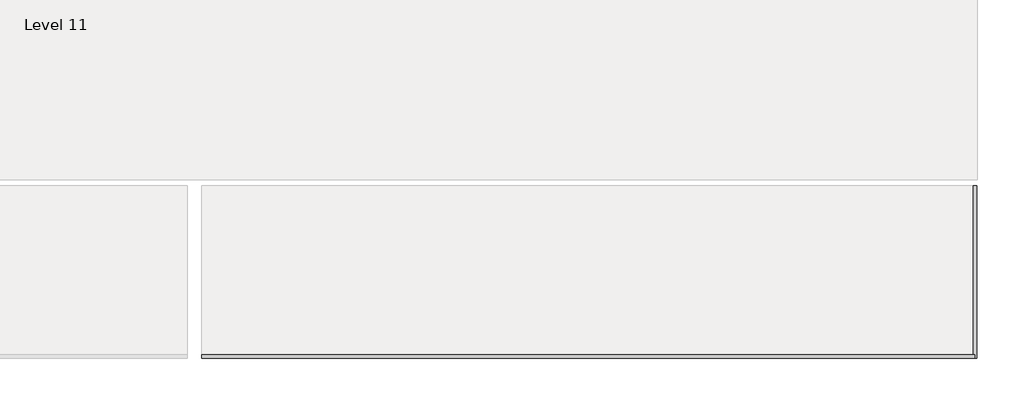
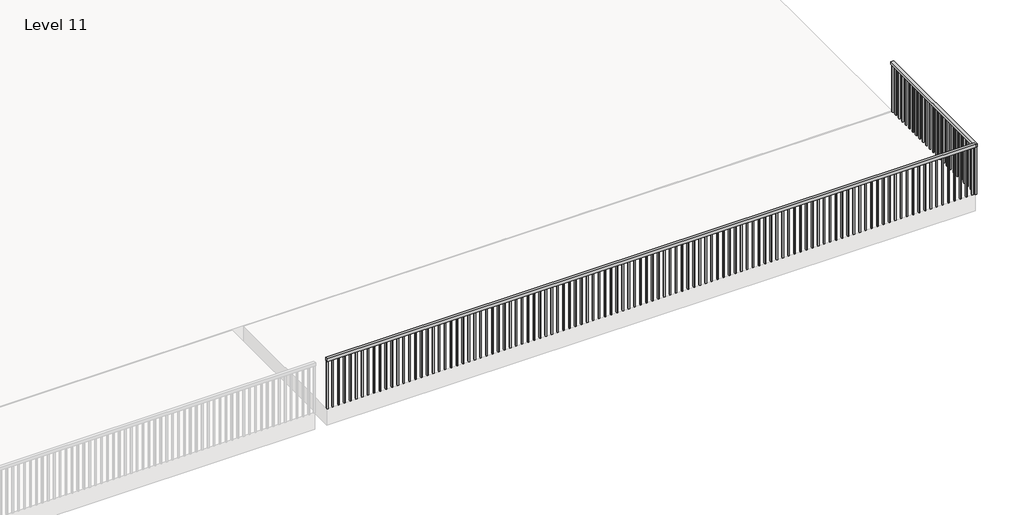
# One storey, part 2 of 5: 2 railings.
"""IFC4 building model written with IfcOpenShell, lengths in millimetres."""

from ifc_helpers import new_model, si_unit, frame, origin, place, context, project, spatial, polyline, outline, extrude, element, save

model = new_model("IFC4")

# Units and contexts
model_context = context("Model", 3, world=origin())
ifc_project = project(units=[si_unit("LENGTHUNIT", "METRE", prefix="MILLI")], contexts=[model_context])

# Site, building, storey
site = spatial("IfcSite", under=ifc_project)
building = spatial("IfcBuilding", under=site)
storey = spatial("IfcBuildingStorey", under=building, Name="Level 11", Elevation=15544.8)

# Railings
placement = place(None, origin())
element("IfcRailing", 1, ObjectType="Handrail - Rectangular", at=placement, inside=storey, context=model_context, shape_type="SweptSolid", body=[
    extrude(outline(polyline([(2981.3361222, -12911.7749501), (2981.3361222, -12860.9749501), (14106.5361222, -12860.9749501), (14106.5361222, -12911.7749501), (2981.3361222, -12911.7749501)])), frame((0.0, 0.0, 16408.4), z_axis=(0.0, 0.0, 1.0), x_axis=(1.0, 0.0, 0.0)), (0.0, 0.0, 1.0), 50.8),
    extrude(outline(polyline([(14046.2111222, -12895.8999501), (14046.2111222, -12876.8499501), (14065.2611222, -12876.8499501), (14065.2611222, -12895.8999501), (14046.2111222, -12895.8999501)])), frame((0.0, 0.0, 15544.8), z_axis=(0.0, 0.0, 1.0), x_axis=(1.0, 0.0, 0.0)), (0.0, 0.0, 1.0), 863.6),
    extrude(outline(polyline([(13944.6111222, -12895.8999501), (13944.6111222, -12876.8499501), (13963.6611222, -12876.8499501), (13963.6611222, -12895.8999501), (13944.6111222, -12895.8999501)])), frame((0.0, 0.0, 15544.8), z_axis=(0.0, 0.0, 1.0), x_axis=(1.0, 0.0, 0.0)), (0.0, 0.0, 1.0), 863.6),
    extrude(outline(polyline([(13843.0111222, -12895.8999501), (13843.0111222, -12876.8499501), (13862.0611222, -12876.8499501), (13862.0611222, -12895.8999501), (13843.0111222, -12895.8999501)])), frame((0.0, 0.0, 15544.8), z_axis=(0.0, 0.0, 1.0), x_axis=(1.0, 0.0, 0.0)), (0.0, 0.0, 1.0), 863.6),
    extrude(outline(polyline([(13741.4111222, -12895.8999501), (13741.4111222, -12876.8499501), (13760.4611222, -12876.8499501), (13760.4611222, -12895.8999501), (13741.4111222, -12895.8999501)])), frame((0.0, 0.0, 15544.8), z_axis=(0.0, 0.0, 1.0), x_axis=(1.0, 0.0, 0.0)), (0.0, 0.0, 1.0), 863.6),
    extrude(outline(polyline([(13639.8111222, -12895.8999501), (13639.8111222, -12876.8499501), (13658.8611222, -12876.8499501), (13658.8611222, -12895.8999501), (13639.8111222, -12895.8999501)])), frame((0.0, 0.0, 15544.8), z_axis=(0.0, 0.0, 1.0), x_axis=(1.0, 0.0, 0.0)), (0.0, 0.0, 1.0), 863.6),
    extrude(outline(polyline([(13538.2111222, -12895.8999501), (13538.2111222, -12876.8499501), (13557.2611222, -12876.8499501), (13557.2611222, -12895.8999501), (13538.2111222, -12895.8999501)])), frame((0.0, 0.0, 15544.8), z_axis=(0.0, 0.0, 1.0), x_axis=(1.0, 0.0, 0.0)), (0.0, 0.0, 1.0), 863.6),
    extrude(outline(polyline([(13436.6111222, -12895.8999501), (13436.6111222, -12876.8499501), (13455.6611222, -12876.8499501), (13455.6611222, -12895.8999501), (13436.6111222, -12895.8999501)])), frame((0.0, 0.0, 15544.8), z_axis=(0.0, 0.0, 1.0), x_axis=(1.0, 0.0, 0.0)), (0.0, 0.0, 1.0), 863.6),
    extrude(outline(polyline([(13335.0111222, -12895.8999501), (13335.0111222, -12876.8499501), (13354.0611222, -12876.8499501), (13354.0611222, -12895.8999501), (13335.0111222, -12895.8999501)])), frame((0.0, 0.0, 15544.8), z_axis=(0.0, 0.0, 1.0), x_axis=(1.0, 0.0, 0.0)), (0.0, 0.0, 1.0), 863.6),
    extrude(outline(polyline([(13233.4111222, -12895.8999501), (13233.4111222, -12876.8499501), (13252.4611222, -12876.8499501), (13252.4611222, -12895.8999501), (13233.4111222, -12895.8999501)])), frame((0.0, 0.0, 15544.8), z_axis=(0.0, 0.0, 1.0), x_axis=(1.0, 0.0, 0.0)), (0.0, 0.0, 1.0), 863.6),
    extrude(outline(polyline([(13131.8111222, -12895.8999501), (13131.8111222, -12876.8499501), (13150.8611222, -12876.8499501), (13150.8611222, -12895.8999501), (13131.8111222, -12895.8999501)])), frame((0.0, 0.0, 15544.8), z_axis=(0.0, 0.0, 1.0), x_axis=(1.0, 0.0, 0.0)), (0.0, 0.0, 1.0), 863.6),
    extrude(outline(polyline([(13030.2111222, -12895.8999501), (13030.2111222, -12876.8499501), (13049.2611222, -12876.8499501), (13049.2611222, -12895.8999501), (13030.2111222, -12895.8999501)])), frame((0.0, 0.0, 15544.8), z_axis=(0.0, 0.0, 1.0), x_axis=(1.0, 0.0, 0.0)), (0.0, 0.0, 1.0), 863.6),
    extrude(outline(polyline([(12928.6111222, -12895.8999501), (12928.6111222, -12876.8499501), (12947.6611222, -12876.8499501), (12947.6611222, -12895.8999501), (12928.6111222, -12895.8999501)])), frame((0.0, 0.0, 15544.8), z_axis=(0.0, 0.0, 1.0), x_axis=(1.0, 0.0, 0.0)), (0.0, 0.0, 1.0), 863.6),
    extrude(outline(polyline([(12827.0111222, -12895.8999501), (12827.0111222, -12876.8499501), (12846.0611222, -12876.8499501), (12846.0611222, -12895.8999501), (12827.0111222, -12895.8999501)])), frame((0.0, 0.0, 15544.8), z_axis=(0.0, 0.0, 1.0), x_axis=(1.0, 0.0, 0.0)), (0.0, 0.0, 1.0), 863.6),
    extrude(outline(polyline([(12725.4111222, -12895.8999501), (12725.4111222, -12876.8499501), (12744.4611222, -12876.8499501), (12744.4611222, -12895.8999501), (12725.4111222, -12895.8999501)])), frame((0.0, 0.0, 15544.8), z_axis=(0.0, 0.0, 1.0), x_axis=(1.0, 0.0, 0.0)), (0.0, 0.0, 1.0), 863.6),
    extrude(outline(polyline([(12623.8111222, -12895.8999501), (12623.8111222, -12876.8499501), (12642.8611222, -12876.8499501), (12642.8611222, -12895.8999501), (12623.8111222, -12895.8999501)])), frame((0.0, 0.0, 15544.8), z_axis=(0.0, 0.0, 1.0), x_axis=(1.0, 0.0, 0.0)), (0.0, 0.0, 1.0), 863.6),
    extrude(outline(polyline([(12522.2111222, -12895.8999501), (12522.2111222, -12876.8499501), (12541.2611222, -12876.8499501), (12541.2611222, -12895.8999501), (12522.2111222, -12895.8999501)])), frame((0.0, 0.0, 15544.8), z_axis=(0.0, 0.0, 1.0), x_axis=(1.0, 0.0, 0.0)), (0.0, 0.0, 1.0), 863.6),
    extrude(outline(polyline([(12420.6111222, -12895.8999501), (12420.6111222, -12876.8499501), (12439.6611222, -12876.8499501), (12439.6611222, -12895.8999501), (12420.6111222, -12895.8999501)])), frame((0.0, 0.0, 15544.8), z_axis=(0.0, 0.0, 1.0), x_axis=(1.0, 0.0, 0.0)), (0.0, 0.0, 1.0), 863.6),
    extrude(outline(polyline([(12319.0111222, -12895.8999501), (12319.0111222, -12876.8499501), (12338.0611222, -12876.8499501), (12338.0611222, -12895.8999501), (12319.0111222, -12895.8999501)])), frame((0.0, 0.0, 15544.8), z_axis=(0.0, 0.0, 1.0), x_axis=(1.0, 0.0, 0.0)), (0.0, 0.0, 1.0), 863.6),
    extrude(outline(polyline([(12217.4111222, -12895.8999501), (12217.4111222, -12876.8499501), (12236.4611222, -12876.8499501), (12236.4611222, -12895.8999501), (12217.4111222, -12895.8999501)])), frame((0.0, 0.0, 15544.8), z_axis=(0.0, 0.0, 1.0), x_axis=(1.0, 0.0, 0.0)), (0.0, 0.0, 1.0), 863.6),
    extrude(outline(polyline([(12115.8111222, -12895.8999501), (12115.8111222, -12876.8499501), (12134.8611222, -12876.8499501), (12134.8611222, -12895.8999501), (12115.8111222, -12895.8999501)])), frame((0.0, 0.0, 15544.8), z_axis=(0.0, 0.0, 1.0), x_axis=(1.0, 0.0, 0.0)), (0.0, 0.0, 1.0), 863.6),
    extrude(outline(polyline([(12014.2111222, -12895.8999501), (12014.2111222, -12876.8499501), (12033.2611222, -12876.8499501), (12033.2611222, -12895.8999501), (12014.2111222, -12895.8999501)])), frame((0.0, 0.0, 15544.8), z_axis=(0.0, 0.0, 1.0), x_axis=(1.0, 0.0, 0.0)), (0.0, 0.0, 1.0), 863.6),
    extrude(outline(polyline([(11912.6111222, -12895.8999501), (11912.6111222, -12876.8499501), (11931.6611222, -12876.8499501), (11931.6611222, -12895.8999501), (11912.6111222, -12895.8999501)])), frame((0.0, 0.0, 15544.8), z_axis=(0.0, 0.0, 1.0), x_axis=(1.0, 0.0, 0.0)), (0.0, 0.0, 1.0), 863.6),
    extrude(outline(polyline([(11811.0111222, -12895.8999501), (11811.0111222, -12876.8499501), (11830.0611222, -12876.8499501), (11830.0611222, -12895.8999501), (11811.0111222, -12895.8999501)])), frame((0.0, 0.0, 15544.8), z_axis=(0.0, 0.0, 1.0), x_axis=(1.0, 0.0, 0.0)), (0.0, 0.0, 1.0), 863.6),
    extrude(outline(polyline([(11709.4111222, -12895.8999501), (11709.4111222, -12876.8499501), (11728.4611222, -12876.8499501), (11728.4611222, -12895.8999501), (11709.4111222, -12895.8999501)])), frame((0.0, 0.0, 15544.8), z_axis=(0.0, 0.0, 1.0), x_axis=(1.0, 0.0, 0.0)), (0.0, 0.0, 1.0), 863.6),
    extrude(outline(polyline([(11607.8111222, -12895.8999501), (11607.8111222, -12876.8499501), (11626.8611222, -12876.8499501), (11626.8611222, -12895.8999501), (11607.8111222, -12895.8999501)])), frame((0.0, 0.0, 15544.8), z_axis=(0.0, 0.0, 1.0), x_axis=(1.0, 0.0, 0.0)), (0.0, 0.0, 1.0), 863.6),
    extrude(outline(polyline([(11506.2111222, -12895.8999501), (11506.2111222, -12876.8499501), (11525.2611222, -12876.8499501), (11525.2611222, -12895.8999501), (11506.2111222, -12895.8999501)])), frame((0.0, 0.0, 15544.8), z_axis=(0.0, 0.0, 1.0), x_axis=(1.0, 0.0, 0.0)), (0.0, 0.0, 1.0), 863.6),
    extrude(outline(polyline([(11404.6111222, -12895.8999501), (11404.6111222, -12876.8499501), (11423.6611222, -12876.8499501), (11423.6611222, -12895.8999501), (11404.6111222, -12895.8999501)])), frame((0.0, 0.0, 15544.8), z_axis=(0.0, 0.0, 1.0), x_axis=(1.0, 0.0, 0.0)), (0.0, 0.0, 1.0), 863.6),
    extrude(outline(polyline([(11303.0111222, -12895.8999501), (11303.0111222, -12876.8499501), (11322.0611222, -12876.8499501), (11322.0611222, -12895.8999501), (11303.0111222, -12895.8999501)])), frame((0.0, 0.0, 15544.8), z_axis=(0.0, 0.0, 1.0), x_axis=(1.0, 0.0, 0.0)), (0.0, 0.0, 1.0), 863.6),
    extrude(outline(polyline([(11201.4111222, -12895.8999501), (11201.4111222, -12876.8499501), (11220.4611222, -12876.8499501), (11220.4611222, -12895.8999501), (11201.4111222, -12895.8999501)])), frame((0.0, 0.0, 15544.8), z_axis=(0.0, 0.0, 1.0), x_axis=(1.0, 0.0, 0.0)), (0.0, 0.0, 1.0), 863.6),
    extrude(outline(polyline([(11099.8111222, -12895.8999501), (11099.8111222, -12876.8499501), (11118.8611222, -12876.8499501), (11118.8611222, -12895.8999501), (11099.8111222, -12895.8999501)])), frame((0.0, 0.0, 15544.8), z_axis=(0.0, 0.0, 1.0), x_axis=(1.0, 0.0, 0.0)), (0.0, 0.0, 1.0), 863.6),
    extrude(outline(polyline([(10998.2111222, -12895.8999501), (10998.2111222, -12876.8499501), (11017.2611222, -12876.8499501), (11017.2611222, -12895.8999501), (10998.2111222, -12895.8999501)])), frame((0.0, 0.0, 15544.8), z_axis=(0.0, 0.0, 1.0), x_axis=(1.0, 0.0, 0.0)), (0.0, 0.0, 1.0), 863.6),
    extrude(outline(polyline([(10896.6111222, -12895.8999501), (10896.6111222, -12876.8499501), (10915.6611222, -12876.8499501), (10915.6611222, -12895.8999501), (10896.6111222, -12895.8999501)])), frame((0.0, 0.0, 15544.8), z_axis=(0.0, 0.0, 1.0), x_axis=(1.0, 0.0, 0.0)), (0.0, 0.0, 1.0), 863.6),
    extrude(outline(polyline([(10795.0111222, -12895.8999501), (10795.0111222, -12876.8499501), (10814.0611222, -12876.8499501), (10814.0611222, -12895.8999501), (10795.0111222, -12895.8999501)])), frame((0.0, 0.0, 15544.8), z_axis=(0.0, 0.0, 1.0), x_axis=(1.0, 0.0, 0.0)), (0.0, 0.0, 1.0), 863.6),
    extrude(outline(polyline([(10693.4111222, -12895.8999501), (10693.4111222, -12876.8499501), (10712.4611222, -12876.8499501), (10712.4611222, -12895.8999501), (10693.4111222, -12895.8999501)])), frame((0.0, 0.0, 15544.8), z_axis=(0.0, 0.0, 1.0), x_axis=(1.0, 0.0, 0.0)), (0.0, 0.0, 1.0), 863.6),
    extrude(outline(polyline([(10591.8111222, -12895.8999501), (10591.8111222, -12876.8499501), (10610.8611222, -12876.8499501), (10610.8611222, -12895.8999501), (10591.8111222, -12895.8999501)])), frame((0.0, 0.0, 15544.8), z_axis=(0.0, 0.0, 1.0), x_axis=(1.0, 0.0, 0.0)), (0.0, 0.0, 1.0), 863.6),
    extrude(outline(polyline([(10490.2111222, -12895.8999501), (10490.2111222, -12876.8499501), (10509.2611222, -12876.8499501), (10509.2611222, -12895.8999501), (10490.2111222, -12895.8999501)])), frame((0.0, 0.0, 15544.8), z_axis=(0.0, 0.0, 1.0), x_axis=(1.0, 0.0, 0.0)), (0.0, 0.0, 1.0), 863.6),
    extrude(outline(polyline([(10388.6111222, -12895.8999501), (10388.6111222, -12876.8499501), (10407.6611222, -12876.8499501), (10407.6611222, -12895.8999501), (10388.6111222, -12895.8999501)])), frame((0.0, 0.0, 15544.8), z_axis=(0.0, 0.0, 1.0), x_axis=(1.0, 0.0, 0.0)), (0.0, 0.0, 1.0), 863.6),
    extrude(outline(polyline([(10287.0111222, -12895.8999501), (10287.0111222, -12876.8499501), (10306.0611222, -12876.8499501), (10306.0611222, -12895.8999501), (10287.0111222, -12895.8999501)])), frame((0.0, 0.0, 15544.8), z_axis=(0.0, 0.0, 1.0), x_axis=(1.0, 0.0, 0.0)), (0.0, 0.0, 1.0), 863.6),
    extrude(outline(polyline([(10185.4111222, -12895.8999501), (10185.4111222, -12876.8499501), (10204.4611222, -12876.8499501), (10204.4611222, -12895.8999501), (10185.4111222, -12895.8999501)])), frame((0.0, 0.0, 15544.8), z_axis=(0.0, 0.0, 1.0), x_axis=(1.0, 0.0, 0.0)), (0.0, 0.0, 1.0), 863.6),
    extrude(outline(polyline([(10083.8111222, -12895.8999501), (10083.8111222, -12876.8499501), (10102.8611222, -12876.8499501), (10102.8611222, -12895.8999501), (10083.8111222, -12895.8999501)])), frame((0.0, 0.0, 15544.8), z_axis=(0.0, 0.0, 1.0), x_axis=(1.0, 0.0, 0.0)), (0.0, 0.0, 1.0), 863.6),
    extrude(outline(polyline([(9982.2111222, -12895.8999501), (9982.2111222, -12876.8499501), (10001.2611222, -12876.8499501), (10001.2611222, -12895.8999501), (9982.2111222, -12895.8999501)])), frame((0.0, 0.0, 15544.8), z_axis=(0.0, 0.0, 1.0), x_axis=(1.0, 0.0, 0.0)), (0.0, 0.0, 1.0), 863.6),
    extrude(outline(polyline([(9880.6111222, -12895.8999501), (9880.6111222, -12876.8499501), (9899.6611222, -12876.8499501), (9899.6611222, -12895.8999501), (9880.6111222, -12895.8999501)])), frame((0.0, 0.0, 15544.8), z_axis=(0.0, 0.0, 1.0), x_axis=(1.0, 0.0, 0.0)), (0.0, 0.0, 1.0), 863.6),
    extrude(outline(polyline([(9779.0111222, -12895.8999501), (9779.0111222, -12876.8499501), (9798.0611222, -12876.8499501), (9798.0611222, -12895.8999501), (9779.0111222, -12895.8999501)])), frame((0.0, 0.0, 15544.8), z_axis=(0.0, 0.0, 1.0), x_axis=(1.0, 0.0, 0.0)), (0.0, 0.0, 1.0), 863.6),
    extrude(outline(polyline([(9677.4111222, -12895.8999501), (9677.4111222, -12876.8499501), (9696.4611222, -12876.8499501), (9696.4611222, -12895.8999501), (9677.4111222, -12895.8999501)])), frame((0.0, 0.0, 15544.8), z_axis=(0.0, 0.0, 1.0), x_axis=(1.0, 0.0, 0.0)), (0.0, 0.0, 1.0), 863.6),
    extrude(outline(polyline([(9575.8111222, -12895.8999501), (9575.8111222, -12876.8499501), (9594.8611222, -12876.8499501), (9594.8611222, -12895.8999501), (9575.8111222, -12895.8999501)])), frame((0.0, 0.0, 15544.8), z_axis=(0.0, 0.0, 1.0), x_axis=(1.0, 0.0, 0.0)), (0.0, 0.0, 1.0), 863.6),
    extrude(outline(polyline([(9474.2111222, -12895.8999501), (9474.2111222, -12876.8499501), (9493.2611222, -12876.8499501), (9493.2611222, -12895.8999501), (9474.2111222, -12895.8999501)])), frame((0.0, 0.0, 15544.8), z_axis=(0.0, 0.0, 1.0), x_axis=(1.0, 0.0, 0.0)), (0.0, 0.0, 1.0), 863.6),
    extrude(outline(polyline([(9372.6111222, -12895.8999501), (9372.6111222, -12876.8499501), (9391.6611222, -12876.8499501), (9391.6611222, -12895.8999501), (9372.6111222, -12895.8999501)])), frame((0.0, 0.0, 15544.8), z_axis=(0.0, 0.0, 1.0), x_axis=(1.0, 0.0, 0.0)), (0.0, 0.0, 1.0), 863.6),
    extrude(outline(polyline([(9271.0111222, -12895.8999501), (9271.0111222, -12876.8499501), (9290.0611222, -12876.8499501), (9290.0611222, -12895.8999501), (9271.0111222, -12895.8999501)])), frame((0.0, 0.0, 15544.8), z_axis=(0.0, 0.0, 1.0), x_axis=(1.0, 0.0, 0.0)), (0.0, 0.0, 1.0), 863.6),
    extrude(outline(polyline([(9169.4111222, -12895.8999501), (9169.4111222, -12876.8499501), (9188.4611222, -12876.8499501), (9188.4611222, -12895.8999501), (9169.4111222, -12895.8999501)])), frame((0.0, 0.0, 15544.8), z_axis=(0.0, 0.0, 1.0), x_axis=(1.0, 0.0, 0.0)), (0.0, 0.0, 1.0), 863.6),
    extrude(outline(polyline([(9067.8111222, -12895.8999501), (9067.8111222, -12876.8499501), (9086.8611222, -12876.8499501), (9086.8611222, -12895.8999501), (9067.8111222, -12895.8999501)])), frame((0.0, 0.0, 15544.8), z_axis=(0.0, 0.0, 1.0), x_axis=(1.0, 0.0, 0.0)), (0.0, 0.0, 1.0), 863.6),
    extrude(outline(polyline([(8966.2111222, -12895.8999501), (8966.2111222, -12876.8499501), (8985.2611222, -12876.8499501), (8985.2611222, -12895.8999501), (8966.2111222, -12895.8999501)])), frame((0.0, 0.0, 15544.8), z_axis=(0.0, 0.0, 1.0), x_axis=(1.0, 0.0, 0.0)), (0.0, 0.0, 1.0), 863.6),
    extrude(outline(polyline([(8864.6111222, -12895.8999501), (8864.6111222, -12876.8499501), (8883.6611222, -12876.8499501), (8883.6611222, -12895.8999501), (8864.6111222, -12895.8999501)])), frame((0.0, 0.0, 15544.8), z_axis=(0.0, 0.0, 1.0), x_axis=(1.0, 0.0, 0.0)), (0.0, 0.0, 1.0), 863.6),
    extrude(outline(polyline([(8763.0111222, -12895.8999501), (8763.0111222, -12876.8499501), (8782.0611222, -12876.8499501), (8782.0611222, -12895.8999501), (8763.0111222, -12895.8999501)])), frame((0.0, 0.0, 15544.8), z_axis=(0.0, 0.0, 1.0), x_axis=(1.0, 0.0, 0.0)), (0.0, 0.0, 1.0), 863.6),
    extrude(outline(polyline([(8661.4111222, -12895.8999501), (8661.4111222, -12876.8499501), (8680.4611222, -12876.8499501), (8680.4611222, -12895.8999501), (8661.4111222, -12895.8999501)])), frame((0.0, 0.0, 15544.8), z_axis=(0.0, 0.0, 1.0), x_axis=(1.0, 0.0, 0.0)), (0.0, 0.0, 1.0), 863.6),
    extrude(outline(polyline([(8559.8111222, -12895.8999501), (8559.8111222, -12876.8499501), (8578.8611222, -12876.8499501), (8578.8611222, -12895.8999501), (8559.8111222, -12895.8999501)])), frame((0.0, 0.0, 15544.8), z_axis=(0.0, 0.0, 1.0), x_axis=(1.0, 0.0, 0.0)), (0.0, 0.0, 1.0), 863.6),
    extrude(outline(polyline([(8458.2111222, -12895.8999501), (8458.2111222, -12876.8499501), (8477.2611222, -12876.8499501), (8477.2611222, -12895.8999501), (8458.2111222, -12895.8999501)])), frame((0.0, 0.0, 15544.8), z_axis=(0.0, 0.0, 1.0), x_axis=(1.0, 0.0, 0.0)), (0.0, 0.0, 1.0), 863.6),
    extrude(outline(polyline([(8356.6111222, -12895.8999501), (8356.6111222, -12876.8499501), (8375.6611222, -12876.8499501), (8375.6611222, -12895.8999501), (8356.6111222, -12895.8999501)])), frame((0.0, 0.0, 15544.8), z_axis=(0.0, 0.0, 1.0), x_axis=(1.0, 0.0, 0.0)), (0.0, 0.0, 1.0), 863.6),
    extrude(outline(polyline([(8255.0111222, -12895.8999501), (8255.0111222, -12876.8499501), (8274.0611222, -12876.8499501), (8274.0611222, -12895.8999501), (8255.0111222, -12895.8999501)])), frame((0.0, 0.0, 15544.8), z_axis=(0.0, 0.0, 1.0), x_axis=(1.0, 0.0, 0.0)), (0.0, 0.0, 1.0), 863.6),
    extrude(outline(polyline([(8153.4111222, -12895.8999501), (8153.4111222, -12876.8499501), (8172.4611222, -12876.8499501), (8172.4611222, -12895.8999501), (8153.4111222, -12895.8999501)])), frame((0.0, 0.0, 15544.8), z_axis=(0.0, 0.0, 1.0), x_axis=(1.0, 0.0, 0.0)), (0.0, 0.0, 1.0), 863.6),
    extrude(outline(polyline([(8051.8111222, -12895.8999501), (8051.8111222, -12876.8499501), (8070.8611222, -12876.8499501), (8070.8611222, -12895.8999501), (8051.8111222, -12895.8999501)])), frame((0.0, 0.0, 15544.8), z_axis=(0.0, 0.0, 1.0), x_axis=(1.0, 0.0, 0.0)), (0.0, 0.0, 1.0), 863.6),
    extrude(outline(polyline([(7950.2111222, -12895.8999501), (7950.2111222, -12876.8499501), (7969.2611222, -12876.8499501), (7969.2611222, -12895.8999501), (7950.2111222, -12895.8999501)])), frame((0.0, 0.0, 15544.8), z_axis=(0.0, 0.0, 1.0), x_axis=(1.0, 0.0, 0.0)), (0.0, 0.0, 1.0), 863.6),
    extrude(outline(polyline([(7848.6111222, -12895.8999501), (7848.6111222, -12876.8499501), (7867.6611222, -12876.8499501), (7867.6611222, -12895.8999501), (7848.6111222, -12895.8999501)])), frame((0.0, 0.0, 15544.8), z_axis=(0.0, 0.0, 1.0), x_axis=(1.0, 0.0, 0.0)), (0.0, 0.0, 1.0), 863.6),
    extrude(outline(polyline([(7747.0111222, -12895.8999501), (7747.0111222, -12876.8499501), (7766.0611222, -12876.8499501), (7766.0611222, -12895.8999501), (7747.0111222, -12895.8999501)])), frame((0.0, 0.0, 15544.8), z_axis=(0.0, 0.0, 1.0), x_axis=(1.0, 0.0, 0.0)), (0.0, 0.0, 1.0), 863.6),
    extrude(outline(polyline([(7645.4111222, -12895.8999501), (7645.4111222, -12876.8499501), (7664.4611222, -12876.8499501), (7664.4611222, -12895.8999501), (7645.4111222, -12895.8999501)])), frame((0.0, 0.0, 15544.8), z_axis=(0.0, 0.0, 1.0), x_axis=(1.0, 0.0, 0.0)), (0.0, 0.0, 1.0), 863.6),
    extrude(outline(polyline([(7543.8111222, -12895.8999501), (7543.8111222, -12876.8499501), (7562.8611222, -12876.8499501), (7562.8611222, -12895.8999501), (7543.8111222, -12895.8999501)])), frame((0.0, 0.0, 15544.8), z_axis=(0.0, 0.0, 1.0), x_axis=(1.0, 0.0, 0.0)), (0.0, 0.0, 1.0), 863.6),
    extrude(outline(polyline([(7442.2111222, -12895.8999501), (7442.2111222, -12876.8499501), (7461.2611222, -12876.8499501), (7461.2611222, -12895.8999501), (7442.2111222, -12895.8999501)])), frame((0.0, 0.0, 15544.8), z_axis=(0.0, 0.0, 1.0), x_axis=(1.0, 0.0, 0.0)), (0.0, 0.0, 1.0), 863.6),
    extrude(outline(polyline([(7340.6111222, -12895.8999501), (7340.6111222, -12876.8499501), (7359.6611222, -12876.8499501), (7359.6611222, -12895.8999501), (7340.6111222, -12895.8999501)])), frame((0.0, 0.0, 15544.8), z_axis=(0.0, 0.0, 1.0), x_axis=(1.0, 0.0, 0.0)), (0.0, 0.0, 1.0), 863.6),
    extrude(outline(polyline([(7239.0111222, -12895.8999501), (7239.0111222, -12876.8499501), (7258.0611222, -12876.8499501), (7258.0611222, -12895.8999501), (7239.0111222, -12895.8999501)])), frame((0.0, 0.0, 15544.8), z_axis=(0.0, 0.0, 1.0), x_axis=(1.0, 0.0, 0.0)), (0.0, 0.0, 1.0), 863.6),
    extrude(outline(polyline([(7137.4111222, -12895.8999501), (7137.4111222, -12876.8499501), (7156.4611222, -12876.8499501), (7156.4611222, -12895.8999501), (7137.4111222, -12895.8999501)])), frame((0.0, 0.0, 15544.8), z_axis=(0.0, 0.0, 1.0), x_axis=(1.0, 0.0, 0.0)), (0.0, 0.0, 1.0), 863.6),
    extrude(outline(polyline([(7035.8111222, -12895.8999501), (7035.8111222, -12876.8499501), (7054.8611222, -12876.8499501), (7054.8611222, -12895.8999501), (7035.8111222, -12895.8999501)])), frame((0.0, 0.0, 15544.8), z_axis=(0.0, 0.0, 1.0), x_axis=(1.0, 0.0, 0.0)), (0.0, 0.0, 1.0), 863.6),
    extrude(outline(polyline([(6934.2111222, -12895.8999501), (6934.2111222, -12876.8499501), (6953.2611222, -12876.8499501), (6953.2611222, -12895.8999501), (6934.2111222, -12895.8999501)])), frame((0.0, 0.0, 15544.8), z_axis=(0.0, 0.0, 1.0), x_axis=(1.0, 0.0, 0.0)), (0.0, 0.0, 1.0), 863.6),
    extrude(outline(polyline([(6832.6111222, -12895.8999501), (6832.6111222, -12876.8499501), (6851.6611222, -12876.8499501), (6851.6611222, -12895.8999501), (6832.6111222, -12895.8999501)])), frame((0.0, 0.0, 15544.8), z_axis=(0.0, 0.0, 1.0), x_axis=(1.0, 0.0, 0.0)), (0.0, 0.0, 1.0), 863.6),
    extrude(outline(polyline([(6731.0111222, -12895.8999501), (6731.0111222, -12876.8499501), (6750.0611222, -12876.8499501), (6750.0611222, -12895.8999501), (6731.0111222, -12895.8999501)])), frame((0.0, 0.0, 15544.8), z_axis=(0.0, 0.0, 1.0), x_axis=(1.0, 0.0, 0.0)), (0.0, 0.0, 1.0), 863.6),
    extrude(outline(polyline([(6629.4111222, -12895.8999501), (6629.4111222, -12876.8499501), (6648.4611222, -12876.8499501), (6648.4611222, -12895.8999501), (6629.4111222, -12895.8999501)])), frame((0.0, 0.0, 15544.8), z_axis=(0.0, 0.0, 1.0), x_axis=(1.0, 0.0, 0.0)), (0.0, 0.0, 1.0), 863.6),
    extrude(outline(polyline([(6527.8111222, -12895.8999501), (6527.8111222, -12876.8499501), (6546.8611222, -12876.8499501), (6546.8611222, -12895.8999501), (6527.8111222, -12895.8999501)])), frame((0.0, 0.0, 15544.8), z_axis=(0.0, 0.0, 1.0), x_axis=(1.0, 0.0, 0.0)), (0.0, 0.0, 1.0), 863.6),
    extrude(outline(polyline([(6426.2111222, -12895.8999501), (6426.2111222, -12876.8499501), (6445.2611222, -12876.8499501), (6445.2611222, -12895.8999501), (6426.2111222, -12895.8999501)])), frame((0.0, 0.0, 15544.8), z_axis=(0.0, 0.0, 1.0), x_axis=(1.0, 0.0, 0.0)), (0.0, 0.0, 1.0), 863.6),
    extrude(outline(polyline([(6324.6111222, -12895.8999501), (6324.6111222, -12876.8499501), (6343.6611222, -12876.8499501), (6343.6611222, -12895.8999501), (6324.6111222, -12895.8999501)])), frame((0.0, 0.0, 15544.8), z_axis=(0.0, 0.0, 1.0), x_axis=(1.0, 0.0, 0.0)), (0.0, 0.0, 1.0), 863.6),
    extrude(outline(polyline([(6223.0111222, -12895.8999501), (6223.0111222, -12876.8499501), (6242.0611222, -12876.8499501), (6242.0611222, -12895.8999501), (6223.0111222, -12895.8999501)])), frame((0.0, 0.0, 15544.8), z_axis=(0.0, 0.0, 1.0), x_axis=(1.0, 0.0, 0.0)), (0.0, 0.0, 1.0), 863.6),
    extrude(outline(polyline([(6121.4111222, -12895.8999501), (6121.4111222, -12876.8499501), (6140.4611222, -12876.8499501), (6140.4611222, -12895.8999501), (6121.4111222, -12895.8999501)])), frame((0.0, 0.0, 15544.8), z_axis=(0.0, 0.0, 1.0), x_axis=(1.0, 0.0, 0.0)), (0.0, 0.0, 1.0), 863.6),
    extrude(outline(polyline([(6019.8111222, -12895.8999501), (6019.8111222, -12876.8499501), (6038.8611222, -12876.8499501), (6038.8611222, -12895.8999501), (6019.8111222, -12895.8999501)])), frame((0.0, 0.0, 15544.8), z_axis=(0.0, 0.0, 1.0), x_axis=(1.0, 0.0, 0.0)), (0.0, 0.0, 1.0), 863.6),
    extrude(outline(polyline([(5918.2111222, -12895.8999501), (5918.2111222, -12876.8499501), (5937.2611222, -12876.8499501), (5937.2611222, -12895.8999501), (5918.2111222, -12895.8999501)])), frame((0.0, 0.0, 15544.8), z_axis=(0.0, 0.0, 1.0), x_axis=(1.0, 0.0, 0.0)), (0.0, 0.0, 1.0), 863.6),
    extrude(outline(polyline([(5816.6111222, -12895.8999501), (5816.6111222, -12876.8499501), (5835.6611222, -12876.8499501), (5835.6611222, -12895.8999501), (5816.6111222, -12895.8999501)])), frame((0.0, 0.0, 15544.8), z_axis=(0.0, 0.0, 1.0), x_axis=(1.0, 0.0, 0.0)), (0.0, 0.0, 1.0), 863.6),
    extrude(outline(polyline([(5715.0111222, -12895.8999501), (5715.0111222, -12876.8499501), (5734.0611222, -12876.8499501), (5734.0611222, -12895.8999501), (5715.0111222, -12895.8999501)])), frame((0.0, 0.0, 15544.8), z_axis=(0.0, 0.0, 1.0), x_axis=(1.0, 0.0, 0.0)), (0.0, 0.0, 1.0), 863.6),
    extrude(outline(polyline([(5613.4111222, -12895.8999501), (5613.4111222, -12876.8499501), (5632.4611222, -12876.8499501), (5632.4611222, -12895.8999501), (5613.4111222, -12895.8999501)])), frame((0.0, 0.0, 15544.8), z_axis=(0.0, 0.0, 1.0), x_axis=(1.0, 0.0, 0.0)), (0.0, 0.0, 1.0), 863.6),
    extrude(outline(polyline([(5511.8111222, -12895.8999501), (5511.8111222, -12876.8499501), (5530.8611222, -12876.8499501), (5530.8611222, -12895.8999501), (5511.8111222, -12895.8999501)])), frame((0.0, 0.0, 15544.8), z_axis=(0.0, 0.0, 1.0), x_axis=(1.0, 0.0, 0.0)), (0.0, 0.0, 1.0), 863.6),
    extrude(outline(polyline([(5410.2111222, -12895.8999501), (5410.2111222, -12876.8499501), (5429.2611222, -12876.8499501), (5429.2611222, -12895.8999501), (5410.2111222, -12895.8999501)])), frame((0.0, 0.0, 15544.8), z_axis=(0.0, 0.0, 1.0), x_axis=(1.0, 0.0, 0.0)), (0.0, 0.0, 1.0), 863.6),
    extrude(outline(polyline([(5308.6111222, -12895.8999501), (5308.6111222, -12876.8499501), (5327.6611222, -12876.8499501), (5327.6611222, -12895.8999501), (5308.6111222, -12895.8999501)])), frame((0.0, 0.0, 15544.8), z_axis=(0.0, 0.0, 1.0), x_axis=(1.0, 0.0, 0.0)), (0.0, 0.0, 1.0), 863.6),
    extrude(outline(polyline([(5207.0111222, -12895.8999501), (5207.0111222, -12876.8499501), (5226.0611222, -12876.8499501), (5226.0611222, -12895.8999501), (5207.0111222, -12895.8999501)])), frame((0.0, 0.0, 15544.8), z_axis=(0.0, 0.0, 1.0), x_axis=(1.0, 0.0, 0.0)), (0.0, 0.0, 1.0), 863.6),
    extrude(outline(polyline([(5105.4111222, -12895.8999501), (5105.4111222, -12876.8499501), (5124.4611222, -12876.8499501), (5124.4611222, -12895.8999501), (5105.4111222, -12895.8999501)])), frame((0.0, 0.0, 15544.8), z_axis=(0.0, 0.0, 1.0), x_axis=(1.0, 0.0, 0.0)), (0.0, 0.0, 1.0), 863.6),
    extrude(outline(polyline([(5003.8111222, -12895.8999501), (5003.8111222, -12876.8499501), (5022.8611222, -12876.8499501), (5022.8611222, -12895.8999501), (5003.8111222, -12895.8999501)])), frame((0.0, 0.0, 15544.8), z_axis=(0.0, 0.0, 1.0), x_axis=(1.0, 0.0, 0.0)), (0.0, 0.0, 1.0), 863.6),
    extrude(outline(polyline([(4902.2111222, -12895.8999501), (4902.2111222, -12876.8499501), (4921.2611222, -12876.8499501), (4921.2611222, -12895.8999501), (4902.2111222, -12895.8999501)])), frame((0.0, 0.0, 15544.8), z_axis=(0.0, 0.0, 1.0), x_axis=(1.0, 0.0, 0.0)), (0.0, 0.0, 1.0), 863.6),
    extrude(outline(polyline([(4800.6111222, -12895.8999501), (4800.6111222, -12876.8499501), (4819.6611222, -12876.8499501), (4819.6611222, -12895.8999501), (4800.6111222, -12895.8999501)])), frame((0.0, 0.0, 15544.8), z_axis=(0.0, 0.0, 1.0), x_axis=(1.0, 0.0, 0.0)), (0.0, 0.0, 1.0), 863.6),
    extrude(outline(polyline([(4699.0111222, -12895.8999501), (4699.0111222, -12876.8499501), (4718.0611222, -12876.8499501), (4718.0611222, -12895.8999501), (4699.0111222, -12895.8999501)])), frame((0.0, 0.0, 15544.8), z_axis=(0.0, 0.0, 1.0), x_axis=(1.0, 0.0, 0.0)), (0.0, 0.0, 1.0), 863.6),
    extrude(outline(polyline([(4597.4111222, -12895.8999501), (4597.4111222, -12876.8499501), (4616.4611222, -12876.8499501), (4616.4611222, -12895.8999501), (4597.4111222, -12895.8999501)])), frame((0.0, 0.0, 15544.8), z_axis=(0.0, 0.0, 1.0), x_axis=(1.0, 0.0, 0.0)), (0.0, 0.0, 1.0), 863.6),
    extrude(outline(polyline([(4495.8111222, -12895.8999501), (4495.8111222, -12876.8499501), (4514.8611222, -12876.8499501), (4514.8611222, -12895.8999501), (4495.8111222, -12895.8999501)])), frame((0.0, 0.0, 15544.8), z_axis=(0.0, 0.0, 1.0), x_axis=(1.0, 0.0, 0.0)), (0.0, 0.0, 1.0), 863.6),
    extrude(outline(polyline([(4394.2111222, -12895.8999501), (4394.2111222, -12876.8499501), (4413.2611222, -12876.8499501), (4413.2611222, -12895.8999501), (4394.2111222, -12895.8999501)])), frame((0.0, 0.0, 15544.8), z_axis=(0.0, 0.0, 1.0), x_axis=(1.0, 0.0, 0.0)), (0.0, 0.0, 1.0), 863.6),
    extrude(outline(polyline([(4292.6111222, -12895.8999501), (4292.6111222, -12876.8499501), (4311.6611222, -12876.8499501), (4311.6611222, -12895.8999501), (4292.6111222, -12895.8999501)])), frame((0.0, 0.0, 15544.8), z_axis=(0.0, 0.0, 1.0), x_axis=(1.0, 0.0, 0.0)), (0.0, 0.0, 1.0), 863.6),
    extrude(outline(polyline([(4191.0111222, -12895.8999501), (4191.0111222, -12876.8499501), (4210.0611222, -12876.8499501), (4210.0611222, -12895.8999501), (4191.0111222, -12895.8999501)])), frame((0.0, 0.0, 15544.8), z_axis=(0.0, 0.0, 1.0), x_axis=(1.0, 0.0, 0.0)), (0.0, 0.0, 1.0), 863.6),
    extrude(outline(polyline([(4089.4111222, -12895.8999501), (4089.4111222, -12876.8499501), (4108.4611222, -12876.8499501), (4108.4611222, -12895.8999501), (4089.4111222, -12895.8999501)])), frame((0.0, 0.0, 15544.8), z_axis=(0.0, 0.0, 1.0), x_axis=(1.0, 0.0, 0.0)), (0.0, 0.0, 1.0), 863.6),
    extrude(outline(polyline([(3987.8111222, -12895.8999501), (3987.8111222, -12876.8499501), (4006.8611222, -12876.8499501), (4006.8611222, -12895.8999501), (3987.8111222, -12895.8999501)])), frame((0.0, 0.0, 15544.8), z_axis=(0.0, 0.0, 1.0), x_axis=(1.0, 0.0, 0.0)), (0.0, 0.0, 1.0), 863.6),
    extrude(outline(polyline([(3886.2111222, -12895.8999501), (3886.2111222, -12876.8499501), (3905.2611222, -12876.8499501), (3905.2611222, -12895.8999501), (3886.2111222, -12895.8999501)])), frame((0.0, 0.0, 15544.8), z_axis=(0.0, 0.0, 1.0), x_axis=(1.0, 0.0, 0.0)), (0.0, 0.0, 1.0), 863.6),
    extrude(outline(polyline([(3784.6111222, -12895.8999501), (3784.6111222, -12876.8499501), (3803.6611222, -12876.8499501), (3803.6611222, -12895.8999501), (3784.6111222, -12895.8999501)])), frame((0.0, 0.0, 15544.8), z_axis=(0.0, 0.0, 1.0), x_axis=(1.0, 0.0, 0.0)), (0.0, 0.0, 1.0), 863.6),
    extrude(outline(polyline([(3683.0111222, -12895.8999501), (3683.0111222, -12876.8499501), (3702.0611222, -12876.8499501), (3702.0611222, -12895.8999501), (3683.0111222, -12895.8999501)])), frame((0.0, 0.0, 15544.8), z_axis=(0.0, 0.0, 1.0), x_axis=(1.0, 0.0, 0.0)), (0.0, 0.0, 1.0), 863.6),
    extrude(outline(polyline([(3581.4111222, -12895.8999501), (3581.4111222, -12876.8499501), (3600.4611222, -12876.8499501), (3600.4611222, -12895.8999501), (3581.4111222, -12895.8999501)])), frame((0.0, 0.0, 15544.8), z_axis=(0.0, 0.0, 1.0), x_axis=(1.0, 0.0, 0.0)), (0.0, 0.0, 1.0), 863.6),
    extrude(outline(polyline([(3479.8111222, -12895.8999501), (3479.8111222, -12876.8499501), (3498.8611222, -12876.8499501), (3498.8611222, -12895.8999501), (3479.8111222, -12895.8999501)])), frame((0.0, 0.0, 15544.8), z_axis=(0.0, 0.0, 1.0), x_axis=(1.0, 0.0, 0.0)), (0.0, 0.0, 1.0), 863.6),
    extrude(outline(polyline([(3378.2111222, -12895.8999501), (3378.2111222, -12876.8499501), (3397.2611222, -12876.8499501), (3397.2611222, -12895.8999501), (3378.2111222, -12895.8999501)])), frame((0.0, 0.0, 15544.8), z_axis=(0.0, 0.0, 1.0), x_axis=(1.0, 0.0, 0.0)), (0.0, 0.0, 1.0), 863.6),
    extrude(outline(polyline([(3276.6111222, -12895.8999501), (3276.6111222, -12876.8499501), (3295.6611222, -12876.8499501), (3295.6611222, -12895.8999501), (3276.6111222, -12895.8999501)])), frame((0.0, 0.0, 15544.8), z_axis=(0.0, 0.0, 1.0), x_axis=(1.0, 0.0, 0.0)), (0.0, 0.0, 1.0), 863.6),
    extrude(outline(polyline([(3175.0111222, -12895.8999501), (3175.0111222, -12876.8499501), (3194.0611222, -12876.8499501), (3194.0611222, -12895.8999501), (3175.0111222, -12895.8999501)])), frame((0.0, 0.0, 15544.8), z_axis=(0.0, 0.0, 1.0), x_axis=(1.0, 0.0, 0.0)), (0.0, 0.0, 1.0), 863.6),
    extrude(outline(polyline([(3073.4111222, -12895.8999501), (3073.4111222, -12876.8499501), (3092.4611222, -12876.8499501), (3092.4611222, -12895.8999501), (3073.4111222, -12895.8999501)])), frame((0.0, 0.0, 15544.8), z_axis=(0.0, 0.0, 1.0), x_axis=(1.0, 0.0, 0.0)), (0.0, 0.0, 1.0), 863.6),
    extrude(outline(polyline([(14087.4861222, -12895.8999501), (14087.4861222, -12876.8499501), (14106.5361222, -12876.8499501), (14106.5361222, -12895.8999501), (14087.4861222, -12895.8999501)])), frame((0.0, 0.0, 15544.8), z_axis=(0.0, 0.0, 1.0), x_axis=(1.0, 0.0, 0.0)), (0.0, 0.0, 1.0), 863.6),
    extrude(outline(polyline([(2981.3361222, -12895.8999501), (2981.3361222, -12876.8499501), (3000.3861222, -12876.8499501), (3000.3861222, -12895.8999501), (2981.3361222, -12895.8999501)])), frame((0.0, 0.0, 15544.8), z_axis=(0.0, 0.0, 1.0), x_axis=(1.0, 0.0, 0.0)), (0.0, 0.0, 1.0), 863.6),
])
element("IfcRailing", 2, ObjectType="Handrail - Rectangular", at=placement, inside=storey, context=model_context, shape_type="SweptSolid", body=[
    extrude(outline(polyline([(14081.1361222, -10428.1762475), (14131.9361222, -10428.1762475), (14131.9361222, -12911.7749501), (14081.1361222, -12911.7749501), (14081.1361222, -10428.1762475)])), frame((0.0, 0.0, 16408.4), z_axis=(0.0, 0.0, 1.0), x_axis=(1.0, 0.0, 0.0)), (0.0, 0.0, 1.0), 50.8),
    extrude(outline(polyline([(14097.0111222, -12857.0512475), (14116.0611222, -12857.0512475), (14116.0611222, -12876.1012475), (14097.0111222, -12876.1012475), (14097.0111222, -12857.0512475)])), frame((0.0, 0.0, 15544.8), z_axis=(0.0, 0.0, 1.0), x_axis=(1.0, 0.0, 0.0)), (0.0, 0.0, 1.0), 863.6),
    extrude(outline(polyline([(14097.0111222, -12755.4512475), (14116.0611222, -12755.4512475), (14116.0611222, -12774.5012475), (14097.0111222, -12774.5012475), (14097.0111222, -12755.4512475)])), frame((0.0, 0.0, 15544.8), z_axis=(0.0, 0.0, 1.0), x_axis=(1.0, 0.0, 0.0)), (0.0, 0.0, 1.0), 863.6),
    extrude(outline(polyline([(14097.0111222, -12653.8512475), (14116.0611222, -12653.8512475), (14116.0611222, -12672.9012475), (14097.0111222, -12672.9012475), (14097.0111222, -12653.8512475)])), frame((0.0, 0.0, 15544.8), z_axis=(0.0, 0.0, 1.0), x_axis=(1.0, 0.0, 0.0)), (0.0, 0.0, 1.0), 863.6),
    extrude(outline(polyline([(14097.0111222, -12552.2512475), (14116.0611222, -12552.2512475), (14116.0611222, -12571.3012475), (14097.0111222, -12571.3012475), (14097.0111222, -12552.2512475)])), frame((0.0, 0.0, 15544.8), z_axis=(0.0, 0.0, 1.0), x_axis=(1.0, 0.0, 0.0)), (0.0, 0.0, 1.0), 863.6),
    extrude(outline(polyline([(14097.0111222, -12450.6512475), (14116.0611222, -12450.6512475), (14116.0611222, -12469.7012475), (14097.0111222, -12469.7012475), (14097.0111222, -12450.6512475)])), frame((0.0, 0.0, 15544.8), z_axis=(0.0, 0.0, 1.0), x_axis=(1.0, 0.0, 0.0)), (0.0, 0.0, 1.0), 863.6),
    extrude(outline(polyline([(14097.0111222, -12349.0512475), (14116.0611222, -12349.0512475), (14116.0611222, -12368.1012475), (14097.0111222, -12368.1012475), (14097.0111222, -12349.0512475)])), frame((0.0, 0.0, 15544.8), z_axis=(0.0, 0.0, 1.0), x_axis=(1.0, 0.0, 0.0)), (0.0, 0.0, 1.0), 863.6),
    extrude(outline(polyline([(14097.0111222, -12247.4512475), (14116.0611222, -12247.4512475), (14116.0611222, -12266.5012475), (14097.0111222, -12266.5012475), (14097.0111222, -12247.4512475)])), frame((0.0, 0.0, 15544.8), z_axis=(0.0, 0.0, 1.0), x_axis=(1.0, 0.0, 0.0)), (0.0, 0.0, 1.0), 863.6),
    extrude(outline(polyline([(14097.0111222, -12145.8512475), (14116.0611222, -12145.8512475), (14116.0611222, -12164.9012475), (14097.0111222, -12164.9012475), (14097.0111222, -12145.8512475)])), frame((0.0, 0.0, 15544.8), z_axis=(0.0, 0.0, 1.0), x_axis=(1.0, 0.0, 0.0)), (0.0, 0.0, 1.0), 863.6),
    extrude(outline(polyline([(14097.0111222, -12044.2512475), (14116.0611222, -12044.2512475), (14116.0611222, -12063.3012475), (14097.0111222, -12063.3012475), (14097.0111222, -12044.2512475)])), frame((0.0, 0.0, 15544.8), z_axis=(0.0, 0.0, 1.0), x_axis=(1.0, 0.0, 0.0)), (0.0, 0.0, 1.0), 863.6),
    extrude(outline(polyline([(14097.0111222, -11942.6512475), (14116.0611222, -11942.6512475), (14116.0611222, -11961.7012475), (14097.0111222, -11961.7012475), (14097.0111222, -11942.6512475)])), frame((0.0, 0.0, 15544.8), z_axis=(0.0, 0.0, 1.0), x_axis=(1.0, 0.0, 0.0)), (0.0, 0.0, 1.0), 863.6),
    extrude(outline(polyline([(14097.0111222, -11841.0512475), (14116.0611222, -11841.0512475), (14116.0611222, -11860.1012475), (14097.0111222, -11860.1012475), (14097.0111222, -11841.0512475)])), frame((0.0, 0.0, 15544.8), z_axis=(0.0, 0.0, 1.0), x_axis=(1.0, 0.0, 0.0)), (0.0, 0.0, 1.0), 863.6),
    extrude(outline(polyline([(14097.0111222, -11739.4512475), (14116.0611222, -11739.4512475), (14116.0611222, -11758.5012475), (14097.0111222, -11758.5012475), (14097.0111222, -11739.4512475)])), frame((0.0, 0.0, 15544.8), z_axis=(0.0, 0.0, 1.0), x_axis=(1.0, 0.0, 0.0)), (0.0, 0.0, 1.0), 863.6),
    extrude(outline(polyline([(14097.0111222, -11637.8512475), (14116.0611222, -11637.8512475), (14116.0611222, -11656.9012475), (14097.0111222, -11656.9012475), (14097.0111222, -11637.8512475)])), frame((0.0, 0.0, 15544.8), z_axis=(0.0, 0.0, 1.0), x_axis=(1.0, 0.0, 0.0)), (0.0, 0.0, 1.0), 863.6),
    extrude(outline(polyline([(14097.0111222, -11536.2512475), (14116.0611222, -11536.2512475), (14116.0611222, -11555.3012475), (14097.0111222, -11555.3012475), (14097.0111222, -11536.2512475)])), frame((0.0, 0.0, 15544.8), z_axis=(0.0, 0.0, 1.0), x_axis=(1.0, 0.0, 0.0)), (0.0, 0.0, 1.0), 863.6),
    extrude(outline(polyline([(14097.0111222, -11434.6512475), (14116.0611222, -11434.6512475), (14116.0611222, -11453.7012475), (14097.0111222, -11453.7012475), (14097.0111222, -11434.6512475)])), frame((0.0, 0.0, 15544.8), z_axis=(0.0, 0.0, 1.0), x_axis=(1.0, 0.0, 0.0)), (0.0, 0.0, 1.0), 863.6),
    extrude(outline(polyline([(14097.0111222, -11333.0512475), (14116.0611222, -11333.0512475), (14116.0611222, -11352.1012475), (14097.0111222, -11352.1012475), (14097.0111222, -11333.0512475)])), frame((0.0, 0.0, 15544.8), z_axis=(0.0, 0.0, 1.0), x_axis=(1.0, 0.0, 0.0)), (0.0, 0.0, 1.0), 863.6),
    extrude(outline(polyline([(14097.0111222, -11231.4512475), (14116.0611222, -11231.4512475), (14116.0611222, -11250.5012475), (14097.0111222, -11250.5012475), (14097.0111222, -11231.4512475)])), frame((0.0, 0.0, 15544.8), z_axis=(0.0, 0.0, 1.0), x_axis=(1.0, 0.0, 0.0)), (0.0, 0.0, 1.0), 863.6),
    extrude(outline(polyline([(14097.0111222, -11129.8512475), (14116.0611222, -11129.8512475), (14116.0611222, -11148.9012475), (14097.0111222, -11148.9012475), (14097.0111222, -11129.8512475)])), frame((0.0, 0.0, 15544.8), z_axis=(0.0, 0.0, 1.0), x_axis=(1.0, 0.0, 0.0)), (0.0, 0.0, 1.0), 863.6),
    extrude(outline(polyline([(14097.0111222, -11028.2512475), (14116.0611222, -11028.2512475), (14116.0611222, -11047.3012475), (14097.0111222, -11047.3012475), (14097.0111222, -11028.2512475)])), frame((0.0, 0.0, 15544.8), z_axis=(0.0, 0.0, 1.0), x_axis=(1.0, 0.0, 0.0)), (0.0, 0.0, 1.0), 863.6),
    extrude(outline(polyline([(14097.0111222, -10926.6512475), (14116.0611222, -10926.6512475), (14116.0611222, -10945.7012475), (14097.0111222, -10945.7012475), (14097.0111222, -10926.6512475)])), frame((0.0, 0.0, 15544.8), z_axis=(0.0, 0.0, 1.0), x_axis=(1.0, 0.0, 0.0)), (0.0, 0.0, 1.0), 863.6),
    extrude(outline(polyline([(14097.0111222, -10825.0512475), (14116.0611222, -10825.0512475), (14116.0611222, -10844.1012475), (14097.0111222, -10844.1012475), (14097.0111222, -10825.0512475)])), frame((0.0, 0.0, 15544.8), z_axis=(0.0, 0.0, 1.0), x_axis=(1.0, 0.0, 0.0)), (0.0, 0.0, 1.0), 863.6),
    extrude(outline(polyline([(14097.0111222, -10723.4512475), (14116.0611222, -10723.4512475), (14116.0611222, -10742.5012475), (14097.0111222, -10742.5012475), (14097.0111222, -10723.4512475)])), frame((0.0, 0.0, 15544.8), z_axis=(0.0, 0.0, 1.0), x_axis=(1.0, 0.0, 0.0)), (0.0, 0.0, 1.0), 863.6),
    extrude(outline(polyline([(14097.0111222, -10621.8512475), (14116.0611222, -10621.8512475), (14116.0611222, -10640.9012475), (14097.0111222, -10640.9012475), (14097.0111222, -10621.8512475)])), frame((0.0, 0.0, 15544.8), z_axis=(0.0, 0.0, 1.0), x_axis=(1.0, 0.0, 0.0)), (0.0, 0.0, 1.0), 863.6),
    extrude(outline(polyline([(14097.0111222, -10520.2512475), (14116.0611222, -10520.2512475), (14116.0611222, -10539.3012475), (14097.0111222, -10539.3012475), (14097.0111222, -10520.2512475)])), frame((0.0, 0.0, 15544.8), z_axis=(0.0, 0.0, 1.0), x_axis=(1.0, 0.0, 0.0)), (0.0, 0.0, 1.0), 863.6),
    extrude(outline(polyline([(14097.0111222, -12892.7249501), (14116.0611222, -12892.7249501), (14116.0611222, -12911.7749501), (14097.0111222, -12911.7749501), (14097.0111222, -12892.7249501)])), frame((0.0, 0.0, 15544.8), z_axis=(0.0, 0.0, 1.0), x_axis=(1.0, 0.0, 0.0)), (0.0, 0.0, 1.0), 863.6),
    extrude(outline(polyline([(14097.0111222, -10428.1762475), (14116.0611222, -10428.1762475), (14116.0611222, -10447.2262475), (14097.0111222, -10447.2262475), (14097.0111222, -10428.1762475)])), frame((0.0, 0.0, 15544.8), z_axis=(0.0, 0.0, 1.0), x_axis=(1.0, 0.0, 0.0)), (0.0, 0.0, 1.0), 863.6),
])

save(model, "model.ifc")

# Revit data of these elements
# Type "Handrail - Rectangular"
#   Assembly Code = "C2010400"
#   built-in parameter 1008612 = 0.0416667 (stored number, unit not read)
#   built-in parameter 1008611 = 0.0416667 (stored number, unit not read)
#   built-in parameter 1008609 = 0.333333 (stored number, unit not read)
#   built-in parameter 1008604 = 0.166667 (stored number, unit not read)
#   built-in parameter 1008603 = 0.166667 (stored number, unit not read)
#   Railing Height = 3' - 0"
#   built-in parameter 1008630 = 2
#   built-in parameter 1008610 = 2
#   built-in parameter 1008618 = Baluster - Square : 3/4"
# Elements 1, 2 (IfcRailing, "Handrail - Rectangular")
#   Phase Created = New Construction
